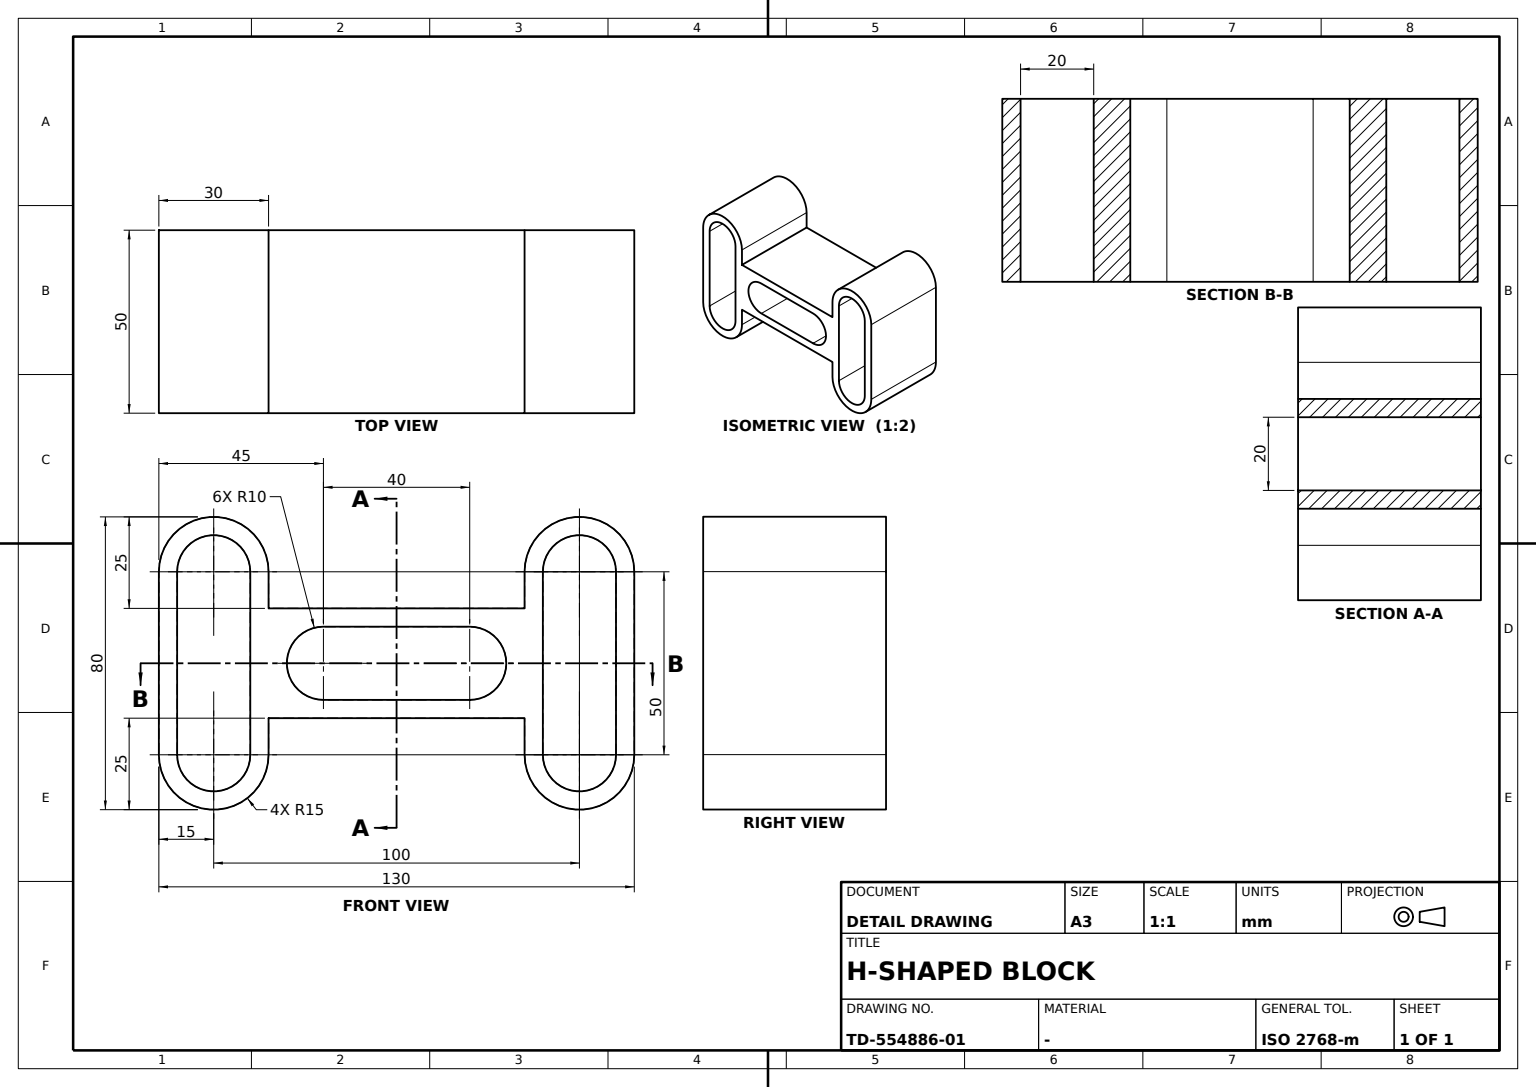
CATIA V5 part; units mm, degrees
sketch "Sketch1" plane through (0, 0, 0) normal (1, 0, 0) x (0, 1, 0)
  line L0 (35, -15) -> (-35, -15)
  line L1 (-35, 15) -> (35, 15)
  point P0 (35, 15)
  point P1 (35, -15)
  point P2 (-35, -15)
  point P3 (-35, 15)
  line L2 (35, 15) -> (35, 25)
  point P4 (35, 25)
  point P5 (65, 25)
  line L3 (65, 25) -> (65, -25)
  point P6 (65, -25)
  point P7 (35, -25)
  line L4 (35, -15) -> (35, -25)
  arc A0 (35, 25) -> (65, 25) centre (50, 25) cw
  point P8 (65, -25)
  point P9 (35, -25)
  arc A1 (35, -25) -> (65, -25) centre (50, -25) ccw
  point P10 (-35, 25)
  point P11 (-35, 15)
  line L5 (-35, 15) -> (-35, 25)
  point P12 (-65, 25)
  arc A2 (-35, 25) -> (-65, 25) centre (-50, 25) ccw
  point P13 (-65, -25)
  line L6 (-65, 25) -> (-65, -25)
  point P14 (-65, -25)
  point P15 (-35, -25)
  arc A3 (-35, -25) -> (-65, -25) centre (-50, -25) cw
  point P16 (-35, -25)
  point P17 (-35, -15)
  line L7 (-35, -15) -> (-35, -25)
  dimension "length L1" = 70
  dimension "length L3" = 50
  dimension "distance P4 P5" = 30
  dimension "distance P0 P1" = 30
  dimension "distance L3 y axis" = 65
  dimension "distance P2 P3" = 30
  dimension "length L7" = 10
  dimension "distance y axis L7" = 35
  constraint horizontal L0 x-axis
  constraint horizontal L1 x-axis
  constraint equidistance L0 L1 origin
  constraint vertical L2 y-axis
  constraint vertical L3 y-axis
  constraint vertical L4 y-axis
  constraint tangency A0 L3
  constraint symmetry P5 P8 x-axis
  constraint symmetry P4 P9 x-axis
  constraint symmetry A0 A1 x-axis
  constraint symmetry P4 P10 y-axis
  constraint symmetry P0 P11 y-axis
  constraint symmetry L2 L5 y-axis
  constraint symmetry P5 P12 y-axis
  constraint symmetry A0 A2 y-axis
  constraint symmetry P6 P13 y-axis
  constraint symmetry L3 L6 y-axis
  constraint symmetry P8 P14 y-axis
  constraint symmetry P9 P15 y-axis
  constraint symmetry A1 A3 y-axis
  constraint symmetry P7 P16 y-axis
  constraint symmetry P1 P17 y-axis
  constraint symmetry L4 L7 y-axis
  constraint coincidence P7 P9
extrude "Pad1" add sketch "Sketch1" along normal mid plane 50
sketch "Sketch2" plane through (0, 0, 0) normal (1, 0, 0) x (0, 1, 0)
  line L0 (20, -10) -> (-20, -10)
  line L1 (-20, 10) -> (20, 10)
  point P0 (20, 10)
  point P1 (20, -10)
  point P2 (-20, -10)
  point P3 (-20, 10)
  arc A0 (20, 10) -> (20, -10) centre (20, 0) cw
  point P4 (-20, -10)
  point P5 (-20, 10)
  arc A1 (-20, 10) -> (-20, -10) centre (-20, 0) ccw
  dimension "length L0" = 40
  dimension "distance P0 P1" = 20
  constraint horizontal L0 x-axis
  constraint horizontal L1 x-axis
  constraint equidistance L0 L1 origin
  constraint tangency A0 L0
  constraint symmetry P1 P4 y-axis
  constraint symmetry P0 P5 y-axis
  constraint symmetry A0 A1 y-axis
  constraint coincidence P2 P4
  constraint coincidence P3 P5
extrude "Pocket1" cut sketch "Sketch2" along normal mid plane 50
sketch "Sketch3" plane through (0, 0, 0) normal (1, 0, 0) x (0, 1, 0)
  point P0 (50, 0)
  arc A0 (60, 25) -> (40, 25) centre (50, 25) ccw
  point P1 (60, 25)
  point P2 (40, 25)
  arc A1 (60, -25) -> (40, -25) centre (50, -25) cw
  point P3 (60, -25)
  point P4 (40, -25)
  line L0 (40, 25) -> (40, -25)
  line L1 (60, 25) -> (60, -25)
  point P5 (-40, -25)
  point P6 (-40, 25)
  line L2 (-40, 25) -> (-40, -25)
  point P7 (-60, -25)
  arc A2 (-60, -25) -> (-40, -25) centre (-50, -25) ccw
  point P8 (-60, 25)
  line L3 (-60, 25) -> (-60, -25)
  arc A3 (-60, 25) -> (-40, 25) centre (-50, 25) cw
  constraint coincidence P0 x-axis
  constraint symmetry A0 A1 x-axis
  constraint symmetry P1 P3 x-axis
  constraint symmetry P2 P4 x-axis
  constraint symmetry P4 P5 y-axis
  constraint symmetry P2 P6 y-axis
  constraint symmetry L0 L2 y-axis
  constraint symmetry P3 P7 y-axis
  constraint symmetry A1 A2 y-axis
  constraint symmetry P1 P8 y-axis
  constraint symmetry L1 L3 y-axis
  constraint symmetry A0 A3 y-axis
  constraint vertical L0 y-axis
  constraint vertical L1 y-axis
extrude "Pocket2" cut sketch "Sketch3" along normal mid plane 50
